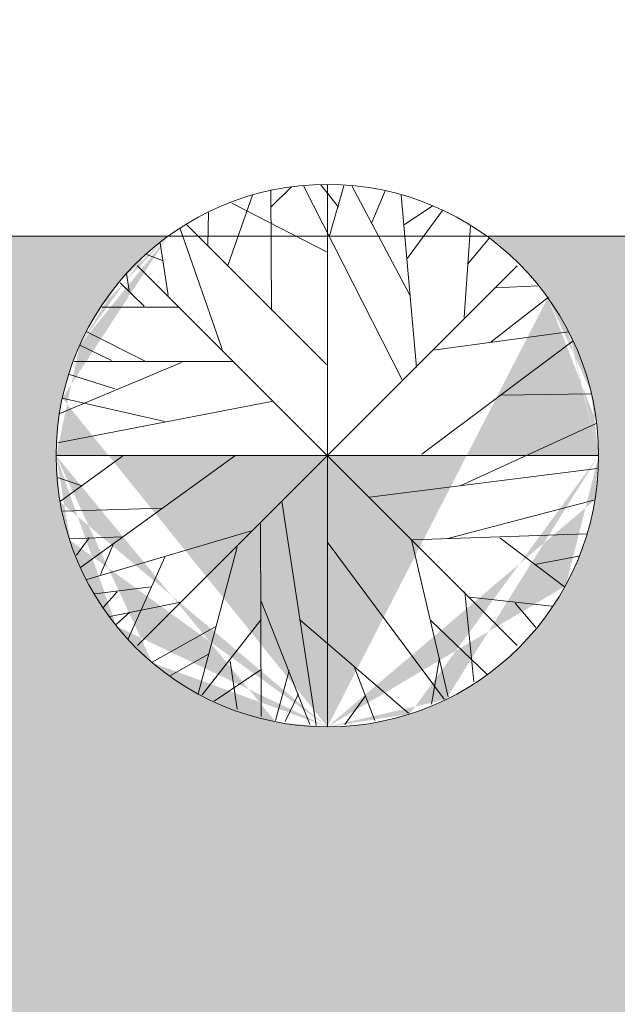
# Model space of a CAD drawing. Units: inches. Extents: x 459864 to 460310, y 324185 to 324787.
# Tile 61 of 112: x 460154 to 460180, y 324239 to 324282. Entities that reach past the tile are written whole.
import ezdxf

# ---------------------------------------------------------------- set-up
doc = ezdxf.new("R2010")
doc.units = ezdxf.units.IN
doc.layers.add('L-PLNT', color=3, linetype='Continuous', lineweight=13)
doc.layers.add('L-SITE-PATT', color=252, linetype='Continuous', lineweight=13)

# ---------------------------------------------------------------- blocks, each defined once
blk = doc.blocks.new('Tree - deciduous plan')
for p, q in [((-12.5388, 54.9406), (-7.9613, 59.4546)), ((-5.3205, 59.6806), (16.5105, 16.7963)), ((2.426, 54.9406), (-1.4472, 59.9056)), ((0, 59.9996), (0, -60)), ((0.4894, 48.6208), (3.6584, 59.6806)), ((18.2711, 35.5298), (5.419, 59.6806)), ((-22.0458, 42.0753), (-16.5881, 57.6486)), ((-12.3627, 32.1443), (-12.5388, 58.7776)), ((9.8203, 51.5549), (12.8133, 58.5516)), ((19.6795, 19.5047), (16.3344, 57.6486)), ((-21.1656, 55.8436), (-0.0388, 45.0094)), ((17.0387, 51.1035), (23.2006, 55.1666)), ((-26.4472, 46.5894), (-26.2712, 53.8116)), ((17.7429, 43.6552), (25.4894, 54.2636)), ((-32.6092, 50.4264), (-23.2782, 23.5674)), ((-31.2008, 51.1035), (-0.2149, 20.1818)), ((31.6513, 50.8778), (30.2429, 30.5643)), ((31.1232, 42.5267), (35.8767, 48.1693)), ((-37.0107, 47.0408), (-35.25, 35.5298)), ((-40.1797, 44.558), (-36.4825, 43.2038)), ((42, 42), (-42, -42)), ((42, -42), (-42, 42)), ((-43.8768, 36.4326), (-44.405, 40.2696)), ((-45.8134, 38.2383), (-40.5318, 33.0471)), ((37.1091, 37.1098), (46.6161, 37.5612)), ((36.2288, 25.1474), (48.9049, 35.0784)), ((-49.8627, 32.8214), (-32.7853, 32.8214)), ((-53.2078, 27.4044), (-40.1797, 20.859)), ((23.3767, 23.3417), (53.3063, 27.4044)), ((-54.7923, 24.4702), (-47.75, 21.0847)), ((54.3626, 25.3731), (20.9119, 0.3198)), ((-32.2571, 20.6333), (-59.1937, 9.348)), ((-56.0247, 20.859), (-20.8134, 20.859)), ((-57.081, 17.9248), (-47.0458, 14.7649)), ((38.5175, 13.4107), (58.2359, 13.6364)), ((-59.7219, 2.8025), (-12.0106, 12.0565)), ((-58.6656, 12.7336), (-35.9543, 7.5424)), ((29.3626, -6.6771), (59.4682, 7.091)), ((-54.6162, -24.7335), (-20.2853, 0.0941)), ((-60, 0), (60, 0)), ((-45.2853, -0.1316), (-59.0177, -10.0627)), ((9.2922, -9.1598), (59.6443, -2.8401)), ((-59.7219, -4.8714), (-54.2641, -6.6771)), ((-10.074, -10.0627), (-2.5036, -59.7178)), ((26.3697, -18.4138), (58.9401, -9.8369)), ((-58.4895, -12.3197), (-36.4825, -11.6426)), ((-14.8275, -15.0282), (-14.6515, -57.6865)), ((-53.2078, -27.442), (-16.7641, -16.6081)), ((18.7992, -18.6394), (57.3556, -17.2853)), ((-57.081, -18.4138), (-45.2853, -17.9624)), ((-52.6797, -18.188), (-55.4966, -22.0251)), ((-47.2219, -19.3166), (-50.2148, -26.3135)), ((-0.0388, -19.0909), (25.8415, -53.8495)), ((18.6232, -18.6394), (26.7218, -53.3981)), ((38.1654, -18.188), (52.426, -29.0219)), ((-19.9331, -20.2194), (-28.5599, -52.721)), ((-35.9543, -22.4765), (-44.0529, -40.5329)), ((45.9119, -24.0564), (55.595, -22.2508)), ((-38.9472, -29.0219), (-51.4472, -30.6018)), ((-46.5177, -30.1504), (-49.5106, -33.536)), ((30.419, -30.1504), (32.3556, -50.0125)), ((-32.4331, -32.4075), (-48.1021, -35.5674)), ((-14.6515, -32.1818), (-3.912, -59.4922)), ((31.4753, -31.279), (49.6091, -33.3103)), ((41.5105, -32.6332), (46.088, -38.0501)), ((-43.7008, -34.6645), (-46.6937, -37.373)), ((-14.6515, -36.2445), (-27.6797, -52.9467)), ((-6.2008, -36.2445), (17.919, -57.0094)), ((22.8485, -36.4702), (35.3485, -48.4326)), ((-24.6867, -37.8244), (-38.7712, -45.7241)), ((-26.2712, -43.9185), (-34.7219, -48.6583)), ((-21.5177, -45.4984), (-19.9331, -56.1065)), ((24.7852, -44.8213), (23.0246, -54.978)), ((-14.6515, -47.3041), (-25.0388, -54.3009)), ((-8.4895, -47.5298), (-11.4825, -58.5893)), ((5.9471, -46.6269), (10.5246, -58.5893)), ((-6.3768, -52.721), (-9.3698, -58.815)), ((8.4119, -53.1724), (3.8344, -59.4922))]:
    blk.add_line(p, q)
blk.add_circle((0, 0), 60)

msp = doc.modelspace()

# ---------------------------------------------------------------- hatches: boundary and pattern name
at = {"layer": 'L-SITE-PATT'}
h = msp.add_hatch(dxfattribs=at)
h.set_pattern_fill('DOTS', color=256)
h.paths.add_polyline_path([(460269.804, 324283.483), (460247.115, 324283.483), (460121.929, 324283.483), (460121.929, 324252.473), (460117.429, 324252.473), (460110.124, 324252.473), (460110.124, 324243.287), (460080.83, 324243.287), (460080.83, 324252.473), (460061.115, 324252.473), (460061.115, 324251.882), (460077.909, 324251.882), (460077.909, 324199.483), (460080.83, 324199.483), (460080.83, 324207.553), (460110.124, 324207.553), (460110.124, 324199.483), (460110.813, 324199.483), (460262.115, 324199.483), (460269.804, 324199.483)], flags=17)
edge = h.paths.add_edge_path(flags=0)
edge.add_ellipse((460222.59, 324263.813), major_axis=(-8.485, 8.485), ratio=1, start_angle=405, end_angle=495, ccw=False)
edge.add_line((460214.821, 324254.66), (460214.832, 324254.666))
edge.add_ellipse((460222.59, 324263.813), major_axis=(-8.485, 8.485), ratio=1, start_angle=405, end_angle=495, ccw=False)
edge.add_line((460210.759, 324261.781), (460210.768, 324261.787))
edge.add_ellipse((460222.59, 324263.813), major_axis=(-8.485, 8.485), ratio=1, start_angle=405, end_angle=495, ccw=False)
edge.add_ellipse((460222.59, 324263.813), major_axis=(-8.485, 8.485), ratio=1, start_angle=392.754, end_angle=405, ccw=False)
edge.add_ellipse((460222.59, 324263.813), major_axis=(-8.485, 8.485), ratio=1, start_angle=380.9347, end_angle=392.754, ccw=False)
edge.add_line((460211.337, 324267.985), (460211.34, 324267.985))
edge.add_ellipse((460222.59, 324263.813), major_axis=(-8.485, 8.485), ratio=1, start_angle=380.9347, end_angle=392.754, ccw=False)
edge.add_ellipse((460222.59, 324263.813), major_axis=(-8.485, 8.485), ratio=1, start_angle=347.9015, end_angle=380.9347, ccw=False)
edge.add_ellipse((460222.59, 324263.813), major_axis=(-8.485, 8.485), ratio=1, start_angle=327.0619, end_angle=347.9015, ccw=False)
edge.add_ellipse((460222.59, 324263.813), major_axis=(-8.485, 8.485), ratio=1, start_angle=278.3246, end_angle=327.0619, ccw=False)
edge.add_line((460225.158, 324275.536), (460225.158, 324275.535))
edge.add_ellipse((460222.59, 324263.813), major_axis=(-8.485, 8.485), ratio=1, start_angle=278.3246, end_angle=327.0619, ccw=False)
edge.add_ellipse((460222.59, 324263.813), major_axis=(-8.485, 8.485), ratio=1, start_angle=260.6436, end_angle=278.3246, ccw=False)
edge.add_ellipse((460222.59, 324263.813), major_axis=(-8.485, 8.485), ratio=1, start_angle=225, end_angle=260.6436, ccw=False)
edge.add_line((460234.509, 324265.243), (460234.501, 324265.239))
edge.add_ellipse((460222.59, 324263.813), major_axis=(-8.485, 8.485), ratio=1, start_angle=225, end_angle=260.6436, ccw=False)
edge.add_ellipse((460222.59, 324263.813), major_axis=(-8.485, 8.485), ratio=1, start_angle=495, end_angle=585, ccw=False)
edge.add_line((460234.437, 324261.861), (460234.424, 324261.858))
edge.add_ellipse((460222.59, 324263.813), major_axis=(-8.485, 8.485), ratio=1, start_angle=495, end_angle=585, ccw=False)
edge.add_line((460227.95, 324253.067), (460227.946, 324253.083))
edge.add_ellipse((460222.59, 324263.813), major_axis=(-8.485, 8.485), ratio=1, start_angle=495, end_angle=585, ccw=False)
edge.add_line((460226.223, 324252.369), (460226.211, 324252.38))
edge.add_ellipse((460222.59, 324263.813), major_axis=(-8.485, 8.485), ratio=1, start_angle=495, end_angle=585, ccw=False)
h.paths.add_polyline_path([(460219.651, 324254.347), (460218.461, 324253.545), (460218.275, 324254.789), (460219.642, 324256.542), (460219.625, 324260.848), (460216.11, 324257.333), (460214.35, 324256.978), (460215.416, 324259.356), (460212.524, 324258.496), (460213.137, 324259.93), (460218.507, 324263.813), (460222.59, 324263.813), (460222.59, 324267.807), (460218.176, 324272.212), (460219.026, 324274.639), (460222.59, 324272.811), (460222.59, 324275.423), (460223.057, 324274.825), (460222.675, 324273.492), (460225.912, 324267.135), (460219.625, 324260.848)], flags=0)
edge = h.paths.add_edge_path(flags=0)
edge.add_ellipse((460194.576, 324264.046), major_axis=(-8.485, 8.485), ratio=1, start_angle=495, end_angle=585, ccw=False)
edge.add_line((460199.936, 324253.3), (460199.932, 324253.316))
edge.add_ellipse((460194.576, 324264.046), major_axis=(-8.485, 8.485), ratio=1, start_angle=495, end_angle=585, ccw=False)
edge.add_line((460198.208, 324252.603), (460198.196, 324252.613))
edge.add_ellipse((460194.576, 324264.046), major_axis=(-8.485, 8.485), ratio=1, start_angle=495, end_angle=585, ccw=False)
edge.add_ellipse((460194.576, 324264.046), major_axis=(-8.485, 8.485), ratio=1, start_angle=405, end_angle=495, ccw=False)
edge.add_line((460186.806, 324254.893), (460186.817, 324254.899))
edge.add_ellipse((460194.576, 324264.046), major_axis=(-8.485, 8.485), ratio=1, start_angle=405, end_angle=495, ccw=False)
edge.add_line((460182.744, 324262.014), (460182.753, 324262.02))
edge.add_ellipse((460194.576, 324264.046), major_axis=(-8.485, 8.485), ratio=1, start_angle=405, end_angle=495, ccw=False)
edge.add_ellipse((460194.576, 324264.046), major_axis=(-8.485, 8.485), ratio=1, start_angle=392.754, end_angle=405, ccw=False)
edge.add_ellipse((460194.576, 324264.046), major_axis=(-8.485, 8.485), ratio=1, start_angle=380.9347, end_angle=392.754, ccw=False)
edge.add_line((460183.323, 324268.218), (460183.326, 324268.218))
edge.add_ellipse((460194.576, 324264.046), major_axis=(-8.485, 8.485), ratio=1, start_angle=380.9347, end_angle=392.754, ccw=False)
edge.add_ellipse((460194.576, 324264.046), major_axis=(-8.485, 8.485), ratio=1, start_angle=347.9015, end_angle=380.9347, ccw=False)
edge.add_ellipse((460194.576, 324264.046), major_axis=(-8.485, 8.485), ratio=1, start_angle=327.0619, end_angle=347.9015, ccw=False)
edge.add_ellipse((460194.576, 324264.046), major_axis=(-8.485, 8.485), ratio=1, start_angle=278.3246, end_angle=327.0619, ccw=False)
edge.add_line((460197.144, 324275.769), (460197.143, 324275.768))
edge.add_ellipse((460194.576, 324264.046), major_axis=(-8.485, 8.485), ratio=1, start_angle=278.3246, end_angle=327.0619, ccw=False)
edge.add_ellipse((460194.576, 324264.046), major_axis=(-8.485, 8.485), ratio=1, start_angle=260.6436, end_angle=278.3246, ccw=False)
edge.add_ellipse((460194.576, 324264.046), major_axis=(-8.485, 8.485), ratio=1, start_angle=225, end_angle=260.6436, ccw=False)
edge.add_line((460206.494, 324265.476), (460206.487, 324265.473))
edge.add_ellipse((460194.576, 324264.046), major_axis=(-8.485, 8.485), ratio=1, start_angle=225, end_angle=260.6436, ccw=False)
edge.add_ellipse((460194.576, 324264.046), major_axis=(-8.485, 8.485), ratio=1, start_angle=495, end_angle=585, ccw=False)
edge.add_line((460206.422, 324262.094), (460206.409, 324262.091))
h.paths.add_polyline_path([(460191.61, 324261.081), (460191.637, 324254.58), (460190.447, 324253.778), (460190.261, 324255.023), (460191.628, 324256.775), (460191.61, 324261.081), (460188.096, 324257.566), (460186.335, 324257.211), (460187.402, 324259.589), (460184.509, 324258.729), (460185.123, 324260.163), (460190.493, 324264.046), (460194.576, 324264.046), (460194.576, 324268.04), (460190.161, 324272.446), (460191.011, 324274.872), (460194.576, 324273.044), (460194.576, 324275.657), (460195.043, 324275.058), (460194.661, 324273.725), (460197.897, 324267.368)], flags=0)
edge = h.paths.add_edge_path(flags=0)
edge.add_ellipse((460252.912, 324263.578), major_axis=(-8.485, 8.485), ratio=1, start_angle=405, end_angle=495, ccw=False)
edge.add_line((460241.081, 324261.545), (460241.089, 324261.551))
edge.add_ellipse((460252.912, 324263.578), major_axis=(-8.485, 8.485), ratio=1, start_angle=405, end_angle=495, ccw=False)
edge.add_ellipse((460252.912, 324263.578), major_axis=(-8.485, 8.485), ratio=1, start_angle=392.754, end_angle=405, ccw=False)
edge.add_ellipse((460252.912, 324263.578), major_axis=(-8.485, 8.485), ratio=1, start_angle=380.9347, end_angle=392.754, ccw=False)
edge.add_line((460241.659, 324267.749), (460241.662, 324267.749))
edge.add_ellipse((460252.912, 324263.578), major_axis=(-8.485, 8.485), ratio=1, start_angle=380.9347, end_angle=392.754, ccw=False)
edge.add_ellipse((460252.912, 324263.578), major_axis=(-8.485, 8.485), ratio=1, start_angle=347.9015, end_angle=380.9347, ccw=False)
edge.add_ellipse((460252.912, 324263.578), major_axis=(-8.485, 8.485), ratio=1, start_angle=327.0619, end_angle=347.9015, ccw=False)
edge.add_ellipse((460252.912, 324263.578), major_axis=(-8.485, 8.485), ratio=1, start_angle=278.3246, end_angle=327.0619, ccw=False)
edge.add_line((460255.48, 324275.3), (460255.479, 324275.299))
edge.add_ellipse((460252.912, 324263.578), major_axis=(-8.485, 8.485), ratio=1, start_angle=278.3246, end_angle=327.0619, ccw=False)
edge.add_ellipse((460252.912, 324263.578), major_axis=(-8.485, 8.485), ratio=1, start_angle=260.6436, end_angle=278.3246, ccw=False)
edge.add_ellipse((460252.912, 324263.578), major_axis=(-8.485, 8.485), ratio=1, start_angle=225, end_angle=260.6436, ccw=False)
edge.add_line((460264.83, 324265.007), (460264.823, 324265.004))
edge.add_ellipse((460252.912, 324263.578), major_axis=(-8.485, 8.485), ratio=1, start_angle=225, end_angle=260.6436, ccw=False)
edge.add_ellipse((460252.912, 324263.578), major_axis=(-8.485, 8.485), ratio=1, start_angle=495, end_angle=585, ccw=False)
edge.add_line((460264.758, 324261.626), (460264.745, 324261.622))
edge.add_ellipse((460252.912, 324263.578), major_axis=(-8.485, 8.485), ratio=1, start_angle=495, end_angle=585, ccw=False)
edge.add_line((460258.272, 324252.832), (460258.268, 324252.848))
edge.add_ellipse((460252.912, 324263.578), major_axis=(-8.485, 8.485), ratio=1, start_angle=495, end_angle=585, ccw=False)
edge.add_line((460256.545, 324252.134), (460256.533, 324252.144))
edge.add_ellipse((460252.912, 324263.578), major_axis=(-8.485, 8.485), ratio=1, start_angle=495, end_angle=585, ccw=False)
edge.add_ellipse((460252.912, 324263.578), major_axis=(-8.485, 8.485), ratio=1, start_angle=405, end_angle=495, ccw=False)
edge.add_line((460245.143, 324254.424), (460245.153, 324254.43))
h.paths.add_polyline_path([(460244.672, 324256.742), (460245.738, 324259.12), (460242.846, 324258.26), (460243.459, 324259.694), (460248.829, 324263.578), (460252.912, 324263.578), (460252.912, 324267.571), (460248.497, 324271.977), (460249.348, 324274.403), (460252.912, 324272.576), (460252.912, 324275.188), (460253.379, 324274.589), (460252.997, 324273.257), (460256.233, 324266.899), (460249.946, 324260.612), (460249.973, 324254.111), (460248.783, 324253.309), (460248.597, 324254.554), (460249.964, 324256.306), (460249.946, 324260.612), (460246.432, 324257.097)], flags=0)
edge = h.paths.add_edge_path(flags=0)
edge.add_ellipse((460167.439, 324262.833), major_axis=(-8.485, 8.485), ratio=1, start_angle=495, end_angle=585, ccw=False)
edge.add_line((460172.799, 324252.087), (460172.795, 324252.103))
edge.add_ellipse((460167.439, 324262.833), major_axis=(-8.485, 8.485), ratio=1, start_angle=495, end_angle=585, ccw=False)
edge.add_line((460171.071, 324251.389), (460171.059, 324251.399))
edge.add_ellipse((460167.439, 324262.833), major_axis=(-8.485, 8.485), ratio=1, start_angle=495, end_angle=585, ccw=False)
edge.add_ellipse((460167.439, 324262.833), major_axis=(-8.485, 8.485), ratio=1, start_angle=405, end_angle=495, ccw=False)
edge.add_line((460159.669, 324253.679), (460159.68, 324253.685))
edge.add_ellipse((460167.439, 324262.833), major_axis=(-8.485, 8.485), ratio=1, start_angle=405, end_angle=495, ccw=False)
edge.add_line((460155.607, 324260.8), (460155.616, 324260.806))
edge.add_ellipse((460167.439, 324262.833), major_axis=(-8.485, 8.485), ratio=1, start_angle=405, end_angle=495, ccw=False)
edge.add_ellipse((460167.439, 324262.833), major_axis=(-8.485, 8.485), ratio=1, start_angle=392.754, end_angle=405, ccw=False)
edge.add_ellipse((460167.439, 324262.833), major_axis=(-8.485, 8.485), ratio=1, start_angle=380.9347, end_angle=392.754, ccw=False)
edge.add_line((460156.185, 324267.005), (460156.189, 324267.005))
edge.add_ellipse((460167.439, 324262.833), major_axis=(-8.485, 8.485), ratio=1, start_angle=380.9347, end_angle=392.754, ccw=False)
edge.add_ellipse((460167.439, 324262.833), major_axis=(-8.485, 8.485), ratio=1, start_angle=347.9015, end_angle=380.9347, ccw=False)
edge.add_ellipse((460167.439, 324262.833), major_axis=(-8.485, 8.485), ratio=1, start_angle=327.0619, end_angle=347.9015, ccw=False)
edge.add_ellipse((460167.439, 324262.833), major_axis=(-8.485, 8.485), ratio=1, start_angle=278.3246, end_angle=327.0619, ccw=False)
edge.add_line((460170.007, 324274.556), (460170.006, 324274.554))
edge.add_ellipse((460167.439, 324262.833), major_axis=(-8.485, 8.485), ratio=1, start_angle=278.3246, end_angle=327.0619, ccw=False)
edge.add_ellipse((460167.439, 324262.833), major_axis=(-8.485, 8.485), ratio=1, start_angle=260.6436, end_angle=278.3246, ccw=False)
edge.add_ellipse((460167.439, 324262.833), major_axis=(-8.485, 8.485), ratio=1, start_angle=225, end_angle=260.6436, ccw=False)
edge.add_line((460179.357, 324264.262), (460179.35, 324264.259))
edge.add_ellipse((460167.439, 324262.833), major_axis=(-8.485, 8.485), ratio=1, start_angle=225, end_angle=260.6436, ccw=False)
edge.add_ellipse((460167.439, 324262.833), major_axis=(-8.485, 8.485), ratio=1, start_angle=495, end_angle=585, ccw=False)
edge.add_line((460179.285, 324260.881), (460179.272, 324260.877))
h.paths.add_polyline_path([(460164.473, 324259.867), (460164.5, 324253.366), (460163.31, 324252.565), (460163.124, 324253.809), (460164.491, 324255.561), (460164.473, 324259.867), (460160.958, 324256.353), (460159.198, 324255.998), (460160.265, 324258.375), (460157.372, 324257.515), (460157.986, 324258.949), (460163.356, 324262.833), (460167.439, 324262.833), (460167.439, 324266.826), (460163.024, 324271.232), (460163.874, 324273.659), (460167.439, 324271.831), (460167.439, 324274.443), (460167.905, 324273.844), (460167.524, 324272.512), (460170.76, 324266.154)], flags=0)
edge = h.paths.add_edge_path(flags=0)
edge.add_ellipse((460140.758, 324262.37), major_axis=(-8.485, 8.485), ratio=1, start_angle=495, end_angle=585, ccw=False)
edge.add_line((460146.118, 324251.624), (460146.114, 324251.639))
edge.add_ellipse((460140.758, 324262.37), major_axis=(-8.485, 8.485), ratio=1, start_angle=495, end_angle=585, ccw=False)
edge.add_line((460144.391, 324250.926), (460144.379, 324250.936))
edge.add_ellipse((460140.758, 324262.37), major_axis=(-8.485, 8.485), ratio=1, start_angle=495, end_angle=585, ccw=False)
edge.add_ellipse((460140.758, 324262.37), major_axis=(-8.485, 8.485), ratio=1, start_angle=405, end_angle=495, ccw=False)
edge.add_line((460132.989, 324253.216), (460132.999, 324253.222))
edge.add_ellipse((460140.758, 324262.37), major_axis=(-8.485, 8.485), ratio=1, start_angle=405, end_angle=495, ccw=False)
edge.add_line((460128.927, 324260.337), (460128.935, 324260.343))
edge.add_ellipse((460140.758, 324262.37), major_axis=(-8.485, 8.485), ratio=1, start_angle=405, end_angle=495, ccw=False)
edge.add_ellipse((460140.758, 324262.37), major_axis=(-8.485, 8.485), ratio=1, start_angle=392.754, end_angle=405, ccw=False)
edge.add_ellipse((460140.758, 324262.37), major_axis=(-8.485, 8.485), ratio=1, start_angle=380.9347, end_angle=392.754, ccw=False)
edge.add_line((460129.505, 324266.541), (460129.508, 324266.541))
edge.add_ellipse((460140.758, 324262.37), major_axis=(-8.485, 8.485), ratio=1, start_angle=380.9347, end_angle=392.754, ccw=False)
edge.add_ellipse((460140.758, 324262.37), major_axis=(-8.485, 8.485), ratio=1, start_angle=347.9015, end_angle=380.9347, ccw=False)
edge.add_ellipse((460140.758, 324262.37), major_axis=(-8.485, 8.485), ratio=1, start_angle=327.0619, end_angle=347.9015, ccw=False)
edge.add_ellipse((460140.758, 324262.37), major_axis=(-8.485, 8.485), ratio=1, start_angle=278.3246, end_angle=327.0619, ccw=False)
edge.add_line((460143.326, 324274.092), (460143.325, 324274.091))
edge.add_ellipse((460140.758, 324262.37), major_axis=(-8.485, 8.485), ratio=1, start_angle=278.3246, end_angle=327.0619, ccw=False)
edge.add_ellipse((460140.758, 324262.37), major_axis=(-8.485, 8.485), ratio=1, start_angle=260.6436, end_angle=278.3246, ccw=False)
edge.add_ellipse((460140.758, 324262.37), major_axis=(-8.485, 8.485), ratio=1, start_angle=225, end_angle=260.6436, ccw=False)
edge.add_line((460152.677, 324263.799), (460152.669, 324263.796))
edge.add_ellipse((460140.758, 324262.37), major_axis=(-8.485, 8.485), ratio=1, start_angle=225, end_angle=260.6436, ccw=False)
edge.add_ellipse((460140.758, 324262.37), major_axis=(-8.485, 8.485), ratio=1, start_angle=495, end_angle=585, ccw=False)
edge.add_line((460152.604, 324260.418), (460152.592, 324260.414))
h.paths.add_polyline_path([(460137.792, 324259.404), (460137.819, 324252.903), (460136.629, 324252.101), (460136.443, 324253.346), (460137.81, 324255.098), (460137.792, 324259.404), (460134.278, 324255.889), (460132.518, 324255.534), (460133.584, 324257.912), (460130.692, 324257.052), (460131.305, 324258.486), (460136.675, 324262.37), (460140.758, 324262.37), (460140.758, 324266.363), (460136.343, 324270.769), (460137.194, 324273.195), (460140.758, 324271.367), (460140.758, 324273.98), (460141.225, 324273.381), (460140.843, 324272.049), (460144.079, 324265.691)], flags=0)
h.paths.add_polyline_path([(460110.124, 324227.414), (460080.83, 324227.414), (460080.83, 324235.484), (460110.124, 324235.484)], flags=16)
h.paths.add_polyline_path([(460110.124, 324220.797), (460110.124, 324212.727), (460080.83, 324212.727), (460080.83, 324220.797)], flags=16)
h.paths.add_polyline_path([(460269.804, 324283.483), (460247.115, 324283.483), (460121.929, 324283.483), (460121.929, 324252.473), (460117.429, 324252.473), (460110.124, 324252.473), (460110.124, 324243.287), (460080.83, 324243.287), (460080.83, 324252.473), (460061.115, 324252.473), (460061.115, 324251.882), (460077.909, 324251.882), (460077.909, 324199.483), (460080.83, 324199.483), (460080.83, 324207.553), (460110.124, 324207.553), (460110.124, 324199.483), (460262.115, 324199.483), (460269.804, 324199.483)], flags=17)
h.paths.add_polyline_path([(460219.651, 324254.347), (460218.461, 324253.545), (460218.275, 324254.789), (460219.642, 324256.542), (460219.625, 324260.848), (460216.11, 324257.333), (460214.35, 324256.978), (460215.416, 324259.356), (460212.524, 324258.496), (460213.137, 324259.93), (460218.507, 324263.813), (460222.59, 324263.813), (460220.18, 324266.223), (460215.461, 324265.308), (460211.835, 324266.137), (460216.247, 324267.985), (460218.418, 324267.985), (460222.59, 324263.813), (460222.59, 324267.807), (460218.176, 324272.212), (460219.026, 324274.639), (460222.59, 324272.811), (460222.59, 324275.423), (460223.057, 324274.825), (460222.675, 324273.492), (460225.912, 324267.135), (460222.59, 324263.813), (460231.383, 324263.813), (460228.485, 324262.488), (460224.425, 324261.978), (460228.68, 324257.724), (460228.966, 324254.791), (460227.142, 324256.537), (460227.542, 324254.819), (460227.333, 324253.614), (460222.59, 324259.985), (460222.59, 324255.497), (460221.377, 324256.541), (460220.576, 324261.799), (460219.625, 324260.848)], flags=0)
h.paths.add_polyline_path([(460199.127, 324256.77), (460199.528, 324255.052), (460199.319, 324253.848), (460194.576, 324260.218), (460194.576, 324255.73), (460193.363, 324256.774), (460192.561, 324262.032), (460191.61, 324261.081), (460191.637, 324254.58), (460190.447, 324253.778), (460190.261, 324255.023), (460191.628, 324256.775), (460191.61, 324261.081), (460188.096, 324257.566), (460186.335, 324257.211), (460187.402, 324259.589), (460184.509, 324258.729), (460185.123, 324260.163), (460190.493, 324264.046), (460194.576, 324264.046), (460192.166, 324266.456), (460187.446, 324265.541), (460183.82, 324266.37), (460188.232, 324268.218), (460190.404, 324268.218), (460194.576, 324264.046), (460194.576, 324268.04), (460190.161, 324272.446), (460191.011, 324274.872), (460194.576, 324273.044), (460194.576, 324275.657), (460195.043, 324275.058), (460194.661, 324273.725), (460197.897, 324267.368), (460194.576, 324264.046), (460203.368, 324264.046), (460200.47, 324262.721), (460196.411, 324262.212), (460200.665, 324257.957), (460200.951, 324255.024)], flags=0)
h.paths.add_polyline_path([(460244.672, 324256.742), (460245.738, 324259.12), (460242.846, 324258.26), (460243.459, 324259.694), (460248.829, 324263.578), (460252.912, 324263.578), (460250.502, 324265.987), (460245.783, 324265.072), (460242.156, 324265.901), (460246.568, 324267.749), (460248.74, 324267.749), (460252.912, 324263.578), (460252.912, 324267.571), (460248.497, 324271.977), (460249.348, 324274.403), (460252.912, 324272.576), (460252.912, 324275.188), (460253.379, 324274.589), (460252.997, 324273.257), (460256.233, 324266.899), (460252.912, 324263.578), (460261.705, 324263.578), (460258.806, 324262.252), (460254.747, 324261.743), (460259.002, 324257.488), (460259.288, 324254.555), (460257.463, 324256.301), (460257.864, 324254.583), (460257.655, 324253.379), (460252.912, 324259.749), (460252.912, 324255.261), (460251.699, 324256.305), (460250.897, 324261.563), (460249.946, 324260.612), (460249.973, 324254.111), (460248.783, 324253.309), (460248.597, 324254.554), (460249.964, 324256.306), (460249.946, 324260.612), (460246.432, 324257.097)], flags=0)
h.paths.add_polyline_path([(460173.528, 324256.743), (460173.814, 324253.811), (460171.99, 324255.556), (460172.39, 324253.838), (460172.182, 324252.634), (460167.439, 324259.004), (460167.439, 324254.516), (460166.226, 324255.56), (460165.424, 324260.818), (460164.473, 324259.867), (460164.5, 324253.366), (460163.31, 324252.565), (460163.124, 324253.809), (460164.491, 324255.561), (460164.473, 324259.867), (460160.958, 324256.353), (460159.198, 324255.998), (460160.265, 324258.375), (460157.372, 324257.515), (460157.986, 324258.949), (460163.356, 324262.833), (460167.439, 324262.833), (460165.029, 324265.243), (460160.309, 324264.327), (460156.683, 324265.156), (460161.095, 324267.005), (460163.267, 324267.005), (460167.439, 324262.833), (460167.439, 324266.826), (460163.024, 324271.232), (460163.874, 324273.659), (460167.439, 324271.831), (460167.439, 324274.443), (460167.905, 324273.844), (460167.524, 324272.512), (460170.76, 324266.154), (460167.439, 324262.833), (460176.231, 324262.833), (460173.333, 324261.507), (460169.274, 324260.998)], flags=0)
h.paths.add_polyline_path([(460146.848, 324256.28), (460147.134, 324253.347), (460145.31, 324255.093), (460145.71, 324253.375), (460145.501, 324252.171), (460140.758, 324258.541), (460140.758, 324254.053), (460139.545, 324255.097), (460138.744, 324260.355), (460137.792, 324259.404), (460137.819, 324252.903), (460136.629, 324252.101), (460136.443, 324253.346), (460137.81, 324255.098), (460137.792, 324259.404), (460134.278, 324255.889), (460132.518, 324255.534), (460133.584, 324257.912), (460130.692, 324257.052), (460131.305, 324258.486), (460136.675, 324262.37), (460140.758, 324262.37), (460138.348, 324264.779), (460133.629, 324263.864), (460130.002, 324264.693), (460134.414, 324266.541), (460136.586, 324266.541), (460140.758, 324262.37), (460140.758, 324266.363), (460136.343, 324270.769), (460137.194, 324273.195), (460140.758, 324271.367), (460140.758, 324273.98), (460141.225, 324273.381), (460140.843, 324272.049), (460144.079, 324265.691), (460140.758, 324262.37), (460149.551, 324262.37), (460146.653, 324261.044), (460142.593, 324260.535)], flags=0)
edge = h.paths.add_edge_path()
edge.add_line((460269.804, 324272.549), (460260.881, 324272.549))
edge.add_ellipse((460252.912, 324263.578), major_axis=(-8.485, 8.485), ratio=1, start_angle=260.6436, end_angle=273.3846, ccw=False)
edge.add_line((460262.283, 324271.092), (460262.261, 324271.091))
edge.add_ellipse((460252.912, 324263.578), major_axis=(-8.485, 8.485), ratio=1, start_angle=260.6436, end_angle=273.3846, ccw=False)
edge.add_ellipse((460252.912, 324263.578), major_axis=(-8.485, 8.485), ratio=1, start_angle=225, end_angle=260.6436, ccw=False)
edge.add_line((460263.609, 324269.063), (460263.572, 324269.058))
edge.add_ellipse((460252.912, 324263.578), major_axis=(-8.485, 8.485), ratio=1, start_angle=225, end_angle=260.6436, ccw=False)
edge.add_line((460264.615, 324266.306), (460264.585, 324266.305))
edge.add_ellipse((460252.912, 324263.578), major_axis=(-8.485, 8.485), ratio=1, start_angle=225, end_angle=260.6436, ccw=False)
edge.add_line((460264.83, 324265.007), (460264.823, 324265.004))
edge.add_ellipse((460252.912, 324263.578), major_axis=(-8.485, 8.485), ratio=1, start_angle=225, end_angle=260.6436, ccw=False)
edge.add_ellipse((460252.912, 324263.578), major_axis=(-8.485, 8.485), ratio=1, start_angle=495, end_angle=585, ccw=False)
edge.add_line((460264.758, 324261.626), (460264.745, 324261.622))
edge.add_ellipse((460252.912, 324263.578), major_axis=(-8.485, 8.485), ratio=1, start_angle=495, end_angle=585, ccw=False)
edge.add_line((460263.442, 324257.739), (460263.389, 324257.779))
edge.add_ellipse((460252.912, 324263.578), major_axis=(-8.485, 8.485), ratio=1, start_angle=495, end_angle=585, ccw=False)
edge.add_line((460258.128, 324252.744), (460258.102, 324252.779))
edge.add_ellipse((460252.912, 324263.578), major_axis=(-8.485, 8.485), ratio=1, start_angle=495, end_angle=585, ccw=False)
edge.add_line((460256.545, 324252.134), (460256.533, 324252.144))
edge.add_ellipse((460252.912, 324263.578), major_axis=(-8.485, 8.485), ratio=1, start_angle=495, end_angle=585, ccw=False)
edge.add_ellipse((460252.912, 324263.578), major_axis=(-8.485, 8.485), ratio=1, start_angle=405, end_angle=495, ccw=False)
edge.add_line((460250.594, 324251.78), (460250.605, 324251.82))
edge.add_ellipse((460252.912, 324263.578), major_axis=(-8.485, 8.485), ratio=1, start_angle=405, end_angle=495, ccw=False)
edge.add_line((460245.143, 324254.424), (460245.153, 324254.43))
edge.add_ellipse((460252.912, 324263.578), major_axis=(-8.485, 8.485), ratio=1, start_angle=405, end_angle=495, ccw=False)
edge.add_line((460243.525, 324256.059), (460243.56, 324256.091))
edge.add_ellipse((460252.912, 324263.578), major_axis=(-8.485, 8.485), ratio=1, start_angle=405, end_angle=495, ccw=False)
edge.add_line((460241.44, 324259.893), (460241.522, 324259.896))
edge.add_ellipse((460252.912, 324263.578), major_axis=(-8.485, 8.485), ratio=1, start_angle=405, end_angle=495, ccw=False)
edge.add_line((460241.081, 324261.545), (460241.089, 324261.551))
edge.add_ellipse((460252.912, 324263.578), major_axis=(-8.485, 8.485), ratio=1, start_angle=405, end_angle=495, ccw=False)
edge.add_ellipse((460252.912, 324263.578), major_axis=(-8.485, 8.485), ratio=1, start_angle=392.754, end_angle=405, ccw=False)
edge.add_line((460241.05, 324265.438), (460241.063, 324265.443))
edge.add_ellipse((460252.912, 324263.578), major_axis=(-8.485, 8.485), ratio=1, start_angle=392.754, end_angle=405, ccw=False)
edge.add_ellipse((460252.912, 324263.578), major_axis=(-8.485, 8.485), ratio=1, start_angle=380.9347, end_angle=392.754, ccw=False)
edge.add_line((460241.452, 324267.176), (460241.469, 324267.171))
edge.add_ellipse((460252.912, 324263.578), major_axis=(-8.485, 8.485), ratio=1, start_angle=380.9347, end_angle=392.754, ccw=False)
edge.add_line((460241.659, 324267.749), (460241.662, 324267.749))
edge.add_ellipse((460252.912, 324263.578), major_axis=(-8.485, 8.485), ratio=1, start_angle=380.9347, end_angle=392.754, ccw=False)
edge.add_ellipse((460252.912, 324263.578), major_axis=(-8.485, 8.485), ratio=1, start_angle=356.6154, end_angle=380.9347, ccw=False)
edge.add_line((460244.88, 324272.488), (460244.713, 324272.549))
edge.add_line((460244.713, 324272.549), (460230.817, 324272.549))
edge.add_ellipse((460222.59, 324263.813), major_axis=(-8.485, 8.485), ratio=1, start_angle=260.6436, end_angle=271.7178, ccw=False)
edge.add_ellipse((460222.59, 324263.813), major_axis=(-8.485, 8.485), ratio=1, start_angle=225, end_angle=260.6436, ccw=False)
edge.add_line((460233.287, 324269.299), (460233.25, 324269.294))
edge.add_ellipse((460222.59, 324263.813), major_axis=(-8.485, 8.485), ratio=1, start_angle=225, end_angle=260.6436, ccw=False)
edge.add_line((460234.294, 324266.541), (460234.264, 324266.541))
edge.add_ellipse((460222.59, 324263.813), major_axis=(-8.485, 8.485), ratio=1, start_angle=225, end_angle=260.6436, ccw=False)
edge.add_line((460234.509, 324265.243), (460234.501, 324265.239))
edge.add_ellipse((460222.59, 324263.813), major_axis=(-8.485, 8.485), ratio=1, start_angle=225, end_angle=260.6436, ccw=False)
edge.add_ellipse((460222.59, 324263.813), major_axis=(-8.485, 8.485), ratio=1, start_angle=495, end_angle=585, ccw=False)
edge.add_line((460234.437, 324261.861), (460234.424, 324261.858))
edge.add_ellipse((460222.59, 324263.813), major_axis=(-8.485, 8.485), ratio=1, start_angle=495, end_angle=585, ccw=False)
edge.add_line((460233.121, 324257.975), (460233.068, 324258.015))
edge.add_ellipse((460222.59, 324263.813), major_axis=(-8.485, 8.485), ratio=1, start_angle=495, end_angle=585, ccw=False)
edge.add_line((460227.806, 324252.979), (460227.78, 324253.014))
edge.add_ellipse((460222.59, 324263.813), major_axis=(-8.485, 8.485), ratio=1, start_angle=495, end_angle=585, ccw=False)
edge.add_line((460226.223, 324252.369), (460226.211, 324252.38))
edge.add_ellipse((460222.59, 324263.813), major_axis=(-8.485, 8.485), ratio=1, start_angle=495, end_angle=585, ccw=False)
edge.add_ellipse((460222.59, 324263.813), major_axis=(-8.485, 8.485), ratio=1, start_angle=405, end_angle=495, ccw=False)
edge.add_line((460220.272, 324252.016), (460220.283, 324252.055))
edge.add_ellipse((460222.59, 324263.813), major_axis=(-8.485, 8.485), ratio=1, start_angle=405, end_angle=495, ccw=False)
edge.add_line((460214.821, 324254.66), (460214.832, 324254.666))
edge.add_ellipse((460222.59, 324263.813), major_axis=(-8.485, 8.485), ratio=1, start_angle=405, end_angle=495, ccw=False)
edge.add_line((460213.203, 324256.295), (460213.239, 324256.327))
edge.add_ellipse((460222.59, 324263.813), major_axis=(-8.485, 8.485), ratio=1, start_angle=405, end_angle=495, ccw=False)
edge.add_line((460211.118, 324260.128), (460211.201, 324260.131))
edge.add_ellipse((460222.59, 324263.813), major_axis=(-8.485, 8.485), ratio=1, start_angle=405, end_angle=495, ccw=False)
edge.add_line((460210.759, 324261.781), (460210.768, 324261.787))
edge.add_ellipse((460222.59, 324263.813), major_axis=(-8.485, 8.485), ratio=1, start_angle=405, end_angle=495, ccw=False)
edge.add_ellipse((460222.59, 324263.813), major_axis=(-8.485, 8.485), ratio=1, start_angle=392.754, end_angle=405, ccw=False)
edge.add_line((460210.729, 324265.673), (460210.741, 324265.678))
edge.add_ellipse((460222.59, 324263.813), major_axis=(-8.485, 8.485), ratio=1, start_angle=392.754, end_angle=405, ccw=False)
edge.add_ellipse((460222.59, 324263.813), major_axis=(-8.485, 8.485), ratio=1, start_angle=380.9347, end_angle=392.754, ccw=False)
edge.add_line((460211.13, 324267.412), (460211.147, 324267.407))
edge.add_ellipse((460222.59, 324263.813), major_axis=(-8.485, 8.485), ratio=1, start_angle=380.9347, end_angle=392.754, ccw=False)
edge.add_line((460211.337, 324267.985), (460211.34, 324267.985))
edge.add_ellipse((460222.59, 324263.813), major_axis=(-8.485, 8.485), ratio=1, start_angle=380.9347, end_angle=392.754, ccw=False)
edge.add_ellipse((460222.59, 324263.813), major_axis=(-8.485, 8.485), ratio=1, start_angle=358.2822, end_angle=380.9347, ccw=False)
edge.add_line((460213.705, 324271.902), (460213.709, 324271.869))
edge.add_ellipse((460222.59, 324263.813), major_axis=(-8.485, 8.485), ratio=1, start_angle=358.2822, end_angle=380.9347, ccw=False)
edge.add_line((460214.363, 324272.549), (460203.078, 324272.549))
edge.add_line((460203.078, 324272.549), (460203.06, 324272.531))
edge.add_ellipse((460194.576, 324264.046), major_axis=(-8.485, 8.485), ratio=1, start_angle=260.6436, end_angle=270.1168, ccw=False)
edge.add_line((460203.957, 324271.561), (460203.921, 324271.56))
edge.add_ellipse((460194.576, 324264.046), major_axis=(-8.485, 8.485), ratio=1, start_angle=260.6436, end_angle=270.1168, ccw=False)
edge.add_ellipse((460194.576, 324264.046), major_axis=(-8.485, 8.485), ratio=1, start_angle=225, end_angle=260.6436, ccw=False)
edge.add_line((460205.272, 324269.532), (460205.235, 324269.527))
edge.add_ellipse((460194.576, 324264.046), major_axis=(-8.485, 8.485), ratio=1, start_angle=225, end_angle=260.6436, ccw=False)
edge.add_line((460206.279, 324266.774), (460206.249, 324266.774))
edge.add_ellipse((460194.576, 324264.046), major_axis=(-8.485, 8.485), ratio=1, start_angle=225, end_angle=260.6436, ccw=False)
edge.add_line((460206.494, 324265.476), (460206.487, 324265.473))
edge.add_ellipse((460194.576, 324264.046), major_axis=(-8.485, 8.485), ratio=1, start_angle=225, end_angle=260.6436, ccw=False)
edge.add_ellipse((460194.576, 324264.046), major_axis=(-8.485, 8.485), ratio=1, start_angle=495, end_angle=585, ccw=False)
edge.add_line((460206.422, 324262.094), (460206.409, 324262.091))
edge.add_ellipse((460194.576, 324264.046), major_axis=(-8.485, 8.485), ratio=1, start_angle=495, end_angle=585, ccw=False)
edge.add_line((460205.106, 324258.208), (460205.053, 324258.248))
edge.add_ellipse((460194.576, 324264.046), major_axis=(-8.485, 8.485), ratio=1, start_angle=495, end_angle=585, ccw=False)
edge.add_line((460199.792, 324253.212), (460199.766, 324253.248))
edge.add_ellipse((460194.576, 324264.046), major_axis=(-8.485, 8.485), ratio=1, start_angle=495, end_angle=585, ccw=False)
edge.add_line((460198.208, 324252.603), (460198.196, 324252.613))
edge.add_ellipse((460194.576, 324264.046), major_axis=(-8.485, 8.485), ratio=1, start_angle=495, end_angle=585, ccw=False)
edge.add_ellipse((460194.576, 324264.046), major_axis=(-8.485, 8.485), ratio=1, start_angle=405, end_angle=495, ccw=False)
edge.add_line((460192.258, 324252.249), (460192.268, 324252.289))
edge.add_ellipse((460194.576, 324264.046), major_axis=(-8.485, 8.485), ratio=1, start_angle=405, end_angle=495, ccw=False)
edge.add_line((460186.806, 324254.893), (460186.817, 324254.899))
edge.add_ellipse((460194.576, 324264.046), major_axis=(-8.485, 8.485), ratio=1, start_angle=405, end_angle=495, ccw=False)
edge.add_line((460185.188, 324256.528), (460185.224, 324256.56))
edge.add_ellipse((460194.576, 324264.046), major_axis=(-8.485, 8.485), ratio=1, start_angle=405, end_angle=495, ccw=False)
edge.add_line((460183.104, 324260.362), (460183.186, 324260.365))
edge.add_ellipse((460194.576, 324264.046), major_axis=(-8.485, 8.485), ratio=1, start_angle=405, end_angle=495, ccw=False)
edge.add_line((460182.744, 324262.014), (460182.753, 324262.02))
edge.add_ellipse((460194.576, 324264.046), major_axis=(-8.485, 8.485), ratio=1, start_angle=405, end_angle=495, ccw=False)
edge.add_ellipse((460194.576, 324264.046), major_axis=(-8.485, 8.485), ratio=1, start_angle=392.754, end_angle=405, ccw=False)
edge.add_line((460182.714, 324265.906), (460182.726, 324265.912))
edge.add_ellipse((460194.576, 324264.046), major_axis=(-8.485, 8.485), ratio=1, start_angle=392.754, end_angle=405, ccw=False)
edge.add_ellipse((460194.576, 324264.046), major_axis=(-8.485, 8.485), ratio=1, start_angle=380.9347, end_angle=392.754, ccw=False)
edge.add_line((460183.116, 324267.645), (460183.133, 324267.64))
edge.add_ellipse((460194.576, 324264.046), major_axis=(-8.485, 8.485), ratio=1, start_angle=380.9347, end_angle=392.754, ccw=False)
edge.add_line((460183.323, 324268.218), (460183.326, 324268.218))
edge.add_ellipse((460194.576, 324264.046), major_axis=(-8.485, 8.485), ratio=1, start_angle=380.9347, end_angle=392.754, ccw=False)
edge.add_ellipse((460194.576, 324264.046), major_axis=(-8.485, 8.485), ratio=1, start_angle=359.8832, end_angle=380.9347, ccw=False)
edge.add_line((460184.491, 324270.611), (460184.553, 324270.611))
edge.add_ellipse((460194.576, 324264.046), major_axis=(-8.485, 8.485), ratio=1, start_angle=359.8832, end_angle=380.9347, ccw=False)
edge.add_line((460185.346, 324271.76), (460185.379, 324271.728))
edge.add_ellipse((460194.576, 324264.046), major_axis=(-8.485, 8.485), ratio=1, start_angle=359.8832, end_angle=380.9347, ccw=False)
edge.add_line((460185.697, 324272.086), (460185.633, 324272.549))
edge.add_line((460185.633, 324272.549), (460174.683, 324272.549))
edge.add_line((460174.683, 324272.549), (460174.606, 324272.457))
edge.add_ellipse((460167.439, 324262.833), major_axis=(-8.485, 8.485), ratio=1, start_angle=260.6436, end_angle=278.3246, ccw=False)
edge.add_ellipse((460167.439, 324262.833), major_axis=(-8.485, 8.485), ratio=1, start_angle=225, end_angle=260.6436, ccw=False)
edge.add_line((460178.135, 324268.318), (460178.098, 324268.313))
edge.add_ellipse((460167.439, 324262.833), major_axis=(-8.485, 8.485), ratio=1, start_angle=225, end_angle=260.6436, ccw=False)
edge.add_line((460179.142, 324265.561), (460179.112, 324265.56))
edge.add_ellipse((460167.439, 324262.833), major_axis=(-8.485, 8.485), ratio=1, start_angle=225, end_angle=260.6436, ccw=False)
edge.add_line((460179.357, 324264.262), (460179.35, 324264.259))
edge.add_ellipse((460167.439, 324262.833), major_axis=(-8.485, 8.485), ratio=1, start_angle=225, end_angle=260.6436, ccw=False)
edge.add_ellipse((460167.439, 324262.833), major_axis=(-8.485, 8.485), ratio=1, start_angle=495, end_angle=585, ccw=False)
edge.add_line((460179.285, 324260.881), (460179.272, 324260.877))
edge.add_ellipse((460167.439, 324262.833), major_axis=(-8.485, 8.485), ratio=1, start_angle=495, end_angle=585, ccw=False)
edge.add_line((460177.969, 324256.994), (460177.916, 324257.034))
edge.add_ellipse((460167.439, 324262.833), major_axis=(-8.485, 8.485), ratio=1, start_angle=495, end_angle=585, ccw=False)
edge.add_line((460172.655, 324251.999), (460172.629, 324252.034))
edge.add_ellipse((460167.439, 324262.833), major_axis=(-8.485, 8.485), ratio=1, start_angle=495, end_angle=585, ccw=False)
edge.add_line((460171.071, 324251.389), (460171.059, 324251.399))
edge.add_ellipse((460167.439, 324262.833), major_axis=(-8.485, 8.485), ratio=1, start_angle=495, end_angle=585, ccw=False)
edge.add_ellipse((460167.439, 324262.833), major_axis=(-8.485, 8.485), ratio=1, start_angle=405, end_angle=495, ccw=False)
edge.add_line((460165.121, 324251.036), (460165.131, 324251.075))
edge.add_ellipse((460167.439, 324262.833), major_axis=(-8.485, 8.485), ratio=1, start_angle=405, end_angle=495, ccw=False)
edge.add_line((460159.669, 324253.679), (460159.68, 324253.685))
edge.add_ellipse((460167.439, 324262.833), major_axis=(-8.485, 8.485), ratio=1, start_angle=405, end_angle=495, ccw=False)
edge.add_line((460158.051, 324255.314), (460158.087, 324255.347))
edge.add_ellipse((460167.439, 324262.833), major_axis=(-8.485, 8.485), ratio=1, start_angle=405, end_angle=495, ccw=False)
edge.add_line((460155.967, 324259.148), (460156.049, 324259.151))
edge.add_ellipse((460167.439, 324262.833), major_axis=(-8.485, 8.485), ratio=1, start_angle=405, end_angle=495, ccw=False)
edge.add_line((460155.607, 324260.8), (460155.616, 324260.806))
edge.add_ellipse((460167.439, 324262.833), major_axis=(-8.485, 8.485), ratio=1, start_angle=405, end_angle=495, ccw=False)
edge.add_ellipse((460167.439, 324262.833), major_axis=(-8.485, 8.485), ratio=1, start_angle=392.754, end_angle=405, ccw=False)
edge.add_line((460155.577, 324264.693), (460155.589, 324264.698))
edge.add_ellipse((460167.439, 324262.833), major_axis=(-8.485, 8.485), ratio=1, start_angle=392.754, end_angle=405, ccw=False)
edge.add_ellipse((460167.439, 324262.833), major_axis=(-8.485, 8.485), ratio=1, start_angle=380.9347, end_angle=392.754, ccw=False)
edge.add_line((460155.979, 324266.432), (460155.996, 324266.426))
edge.add_ellipse((460167.439, 324262.833), major_axis=(-8.485, 8.485), ratio=1, start_angle=380.9347, end_angle=392.754, ccw=False)
edge.add_line((460156.185, 324267.005), (460156.189, 324267.005))
edge.add_ellipse((460167.439, 324262.833), major_axis=(-8.485, 8.485), ratio=1, start_angle=380.9347, end_angle=392.754, ccw=False)
edge.add_ellipse((460167.439, 324262.833), major_axis=(-8.485, 8.485), ratio=1, start_angle=350.9345, end_angle=380.9347, ccw=False)
edge.add_line((460157.363, 324269.397), (460157.414, 324269.397))
edge.add_ellipse((460167.439, 324262.833), major_axis=(-8.485, 8.485), ratio=1, start_angle=350.9345, end_angle=380.9347, ccw=False)
edge.add_line((460158.221, 324270.535), (460158.236, 324270.519))
edge.add_ellipse((460167.439, 324262.833), major_axis=(-8.485, 8.485), ratio=1, start_angle=350.9345, end_angle=380.9347, ccw=False)
edge.add_line((460159.379, 324271.753), (460159.419, 324271.738))
edge.add_ellipse((460167.439, 324262.833), major_axis=(-8.485, 8.485), ratio=1, start_angle=350.9345, end_angle=380.9347, ccw=False)
edge.add_line((460160.396, 324272.549), (460147.112, 324272.549))
edge.add_ellipse((460140.758, 324262.37), major_axis=(-8.485, 8.485), ratio=1, start_angle=278.3246, end_angle=283.0261, ccw=False)
edge.add_ellipse((460140.758, 324262.37), major_axis=(-8.485, 8.485), ratio=1, start_angle=260.6436, end_angle=278.3246, ccw=False)
edge.add_ellipse((460140.758, 324262.37), major_axis=(-8.485, 8.485), ratio=1, start_angle=225, end_angle=260.6436, ccw=False)
edge.add_line((460151.455, 324267.855), (460151.418, 324267.85))
edge.add_ellipse((460140.758, 324262.37), major_axis=(-8.485, 8.485), ratio=1, start_angle=225, end_angle=260.6436, ccw=False)
edge.add_line((460152.462, 324265.098), (460152.431, 324265.097))
edge.add_ellipse((460140.758, 324262.37), major_axis=(-8.485, 8.485), ratio=1, start_angle=225, end_angle=260.6436, ccw=False)
edge.add_line((460152.677, 324263.799), (460152.669, 324263.796))
edge.add_ellipse((460140.758, 324262.37), major_axis=(-8.485, 8.485), ratio=1, start_angle=225, end_angle=260.6436, ccw=False)
edge.add_ellipse((460140.758, 324262.37), major_axis=(-8.485, 8.485), ratio=1, start_angle=495, end_angle=585, ccw=False)
edge.add_line((460152.604, 324260.418), (460152.592, 324260.414))
edge.add_ellipse((460140.758, 324262.37), major_axis=(-8.485, 8.485), ratio=1, start_angle=495, end_angle=585, ccw=False)
edge.add_line((460151.288, 324256.531), (460151.235, 324256.571))
edge.add_ellipse((460140.758, 324262.37), major_axis=(-8.485, 8.485), ratio=1, start_angle=495, end_angle=585, ccw=False)
edge.add_line((460145.974, 324251.535), (460145.948, 324251.571))
edge.add_ellipse((460140.758, 324262.37), major_axis=(-8.485, 8.485), ratio=1, start_angle=495, end_angle=585, ccw=False)
edge.add_line((460144.391, 324250.926), (460144.379, 324250.936))
edge.add_ellipse((460140.758, 324262.37), major_axis=(-8.485, 8.485), ratio=1, start_angle=495, end_angle=585, ccw=False)
edge.add_ellipse((460140.758, 324262.37), major_axis=(-8.485, 8.485), ratio=1, start_angle=405, end_angle=495, ccw=False)
edge.add_line((460138.44, 324250.572), (460138.451, 324250.612))
edge.add_ellipse((460140.758, 324262.37), major_axis=(-8.485, 8.485), ratio=1, start_angle=405, end_angle=495, ccw=False)
edge.add_line((460132.989, 324253.216), (460132.999, 324253.222))
edge.add_ellipse((460140.758, 324262.37), major_axis=(-8.485, 8.485), ratio=1, start_angle=405, end_angle=495, ccw=False)
edge.add_line((460131.371, 324254.851), (460131.406, 324254.883))
edge.add_ellipse((460140.758, 324262.37), major_axis=(-8.485, 8.485), ratio=1, start_angle=405, end_angle=495, ccw=False)
edge.add_line((460129.286, 324258.685), (460129.369, 324258.688))
edge.add_ellipse((460140.758, 324262.37), major_axis=(-8.485, 8.485), ratio=1, start_angle=405, end_angle=495, ccw=False)
edge.add_line((460128.927, 324260.337), (460128.935, 324260.343))
edge.add_ellipse((460140.758, 324262.37), major_axis=(-8.485, 8.485), ratio=1, start_angle=405, end_angle=495, ccw=False)
edge.add_ellipse((460140.758, 324262.37), major_axis=(-8.485, 8.485), ratio=1, start_angle=392.754, end_angle=405, ccw=False)
edge.add_line((460128.896, 324264.23), (460128.909, 324264.235))
edge.add_ellipse((460140.758, 324262.37), major_axis=(-8.485, 8.485), ratio=1, start_angle=392.754, end_angle=405, ccw=False)
edge.add_ellipse((460140.758, 324262.37), major_axis=(-8.485, 8.485), ratio=1, start_angle=380.9347, end_angle=392.754, ccw=False)
edge.add_line((460129.298, 324265.968), (460129.315, 324265.963))
edge.add_ellipse((460140.758, 324262.37), major_axis=(-8.485, 8.485), ratio=1, start_angle=380.9347, end_angle=392.754, ccw=False)
edge.add_line((460129.505, 324266.541), (460129.508, 324266.541))
edge.add_ellipse((460140.758, 324262.37), major_axis=(-8.485, 8.485), ratio=1, start_angle=380.9347, end_angle=392.754, ccw=False)
edge.add_ellipse((460140.758, 324262.37), major_axis=(-8.485, 8.485), ratio=1, start_angle=347.9015, end_angle=380.9347, ccw=False)
edge.add_line((460130.697, 324268.934), (460130.727, 324268.934))
edge.add_ellipse((460140.758, 324262.37), major_axis=(-8.485, 8.485), ratio=1, start_angle=347.9015, end_angle=380.9347, ccw=False)
edge.add_line((460131.869, 324270.48), (460131.879, 324270.413))
edge.add_ellipse((460140.758, 324262.37), major_axis=(-8.485, 8.485), ratio=1, start_angle=347.9015, end_angle=380.9347, ccw=False)
edge.add_line((460132.734, 324271.277), (460132.705, 324271.287))
edge.add_ellipse((460140.758, 324262.37), major_axis=(-8.485, 8.485), ratio=1, start_angle=347.9015, end_angle=380.9347, ccw=False)
edge.add_line((460134.24, 324272.445), (460134.204, 324272.549))
edge.add_line((460134.204, 324272.549), (460121.929, 324272.549))
edge.add_line((460121.929, 324272.549), (460121.929, 324252.473))
edge.add_line((460121.929, 324252.473), (460117.429, 324252.473))
edge.add_line((460117.429, 324252.473), (460110.124, 324252.473))
edge.add_line((460110.124, 324252.473), (460110.124, 324243.287))
edge.add_line((460110.124, 324243.287), (460080.83, 324243.287))
edge.add_line((460080.83, 324243.287), (460080.83, 324252.473))
edge.add_line((460080.83, 324252.473), (460061.115, 324252.473))
edge.add_line((460061.115, 324252.473), (460061.115, 324251.882))
edge.add_line((460061.115, 324251.882), (460077.909, 324251.882))
edge.add_line((460077.909, 324251.882), (460077.909, 324199.483))
edge.add_line((460077.909, 324199.483), (460080.83, 324199.483))
edge.add_line((460080.83, 324199.483), (460080.83, 324207.553))
edge.add_line((460080.83, 324207.553), (460110.124, 324207.553))
edge.add_line((460110.124, 324207.553), (460110.124, 324199.483))
edge.add_line((460110.124, 324199.483), (460110.813, 324199.483))
edge.add_line((460110.813, 324199.483), (460262.115, 324199.483))
edge.add_line((460262.115, 324199.483), (460269.804, 324199.483))
edge.add_line((460269.804, 324199.483), (460269.804, 324272.549))

# ---------------------------------------------------------------- linework, layer by layer
at = {"layer": 'L-PLNT'}
msp.add_line((460121.929, 324272.549), (460269.804, 324272.549), dxfattribs=at)

# ---------------------------------------------------------------- block references
at = {"layer": 'L-PLNT', "xscale": 0.2, "yscale": 0.2}
msp.add_blockref('Tree - deciduous plan', (460167.439, 324262.833), dxfattribs=at)

doc.saveas('drawing.dxf')
